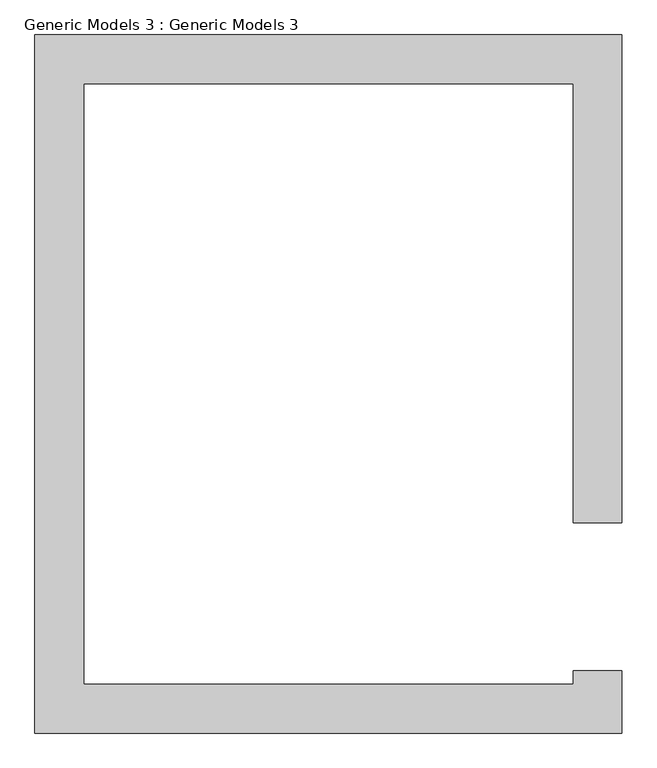
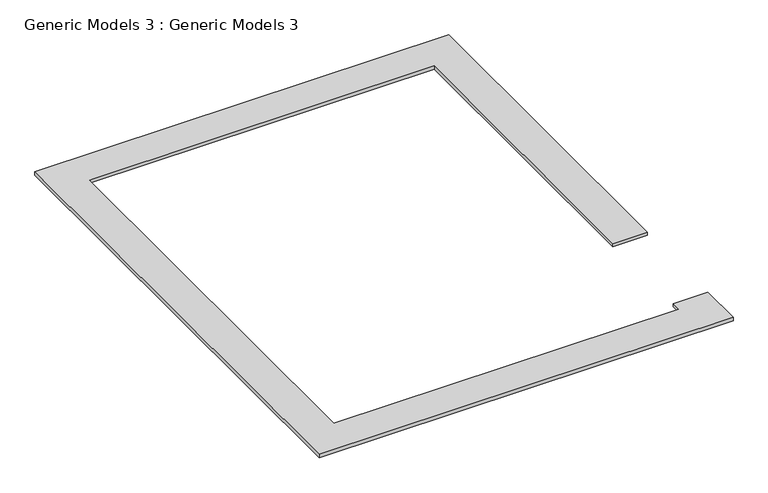
"""IFC4 building model written with IfcOpenShell, lengths in millimetres: proxy geometry, Generic Models 3 : Generic Models 3."""

from ifc_helpers import new_model, si_unit, frame, origin, place, context, project, spatial, polyline, outline, extrude, source, transform, mapped, element, save


def generic_models_3_generic_models_3_9cf6d621(model_context):
    return source(origin(), model_context, "Body", "SweptSolid", [
        extrude(outline(polyline([(-12589.2277598, -4668.8657199), (1698.2722402, -4668.8657199), (1698.2722402, -4275.1657199), (3120.6722402, -4275.1657199), (3120.6722402, -6091.2657199), (-14011.6277598, -6091.2657199), (-14011.6277598, 14292.2342801), (3120.6722402, 14292.2342801), (3120.6722402, 55.5342801), (1698.2722402, 55.5342801), (1698.2722402, 12869.8342801), (-12589.2277598, 12869.8342801), (-12589.2277598, -4668.8657199)])), frame((0.0, 0.0, -135.586224), z_axis=(0.0, 0.0, 1.0), x_axis=(1.0, 0.0, 0.0)), (0.0, 0.0, 1.0), 139.8928993),
    ])


if __name__ == "__main__":
    model = new_model("IFC4")
    model_context = context("Model", 3, world=origin())
    ifc_project = project(units=[si_unit("LENGTHUNIT", "METRE", prefix="MILLI")], contexts=[model_context])
    site = spatial("IfcSite", under=ifc_project)
    building = spatial("IfcBuilding", under=site)
    placement = place(None, origin())
    generic_models_3_generic_models_3_shape = generic_models_3_generic_models_3_9cf6d621(model_context)
    element("IfcBuildingElementProxy", 1, Name="Generic Models 3 : Generic Models 3", ObjectType="Generic Models 3 : Generic Models 3", at=placement, inside=building, context=model_context, shape_type="MappedRepresentation", body=[
        mapped(generic_models_3_generic_models_3_shape, transform((0.0, 0.0, 0.0), x_axis=(1.0, 0.0, 0.0), y_axis=(0.0, 1.0, 0.0), z_axis=(0.0, 0.0, 1.0))),
    ])
    save(model, "model.ifc")

# Revit data of these elements
# Element 1 (IfcBuildingElementProxy, "Generic Models 3 : Generic Models 3")
#   Materials on its faces: "Earth"
# Materials
#   "Earth": class "Generic", colour RGB 44 28 16, transparency 0, Description = "Soil", Cost = 0
